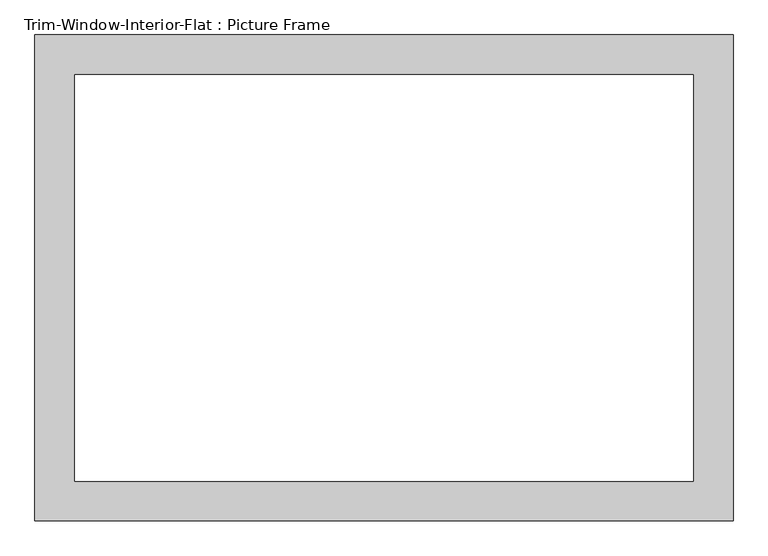
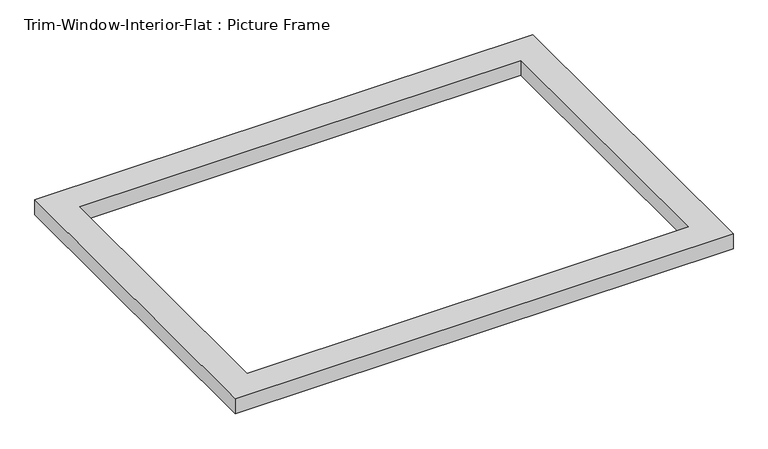
"""IFC4 building model written with IfcOpenShell, lengths in millimetres: proxy geometry, Trim-Window-Interior-Flat : Picture Frame."""

from ifc_helpers import new_model, si_unit, origin, origin_with_axes, place, context, project, spatial, polyline, outline, extrude, source, transform, mapped, element, save


def trim_window_interior_flat_picture_frame_6592d821(model_context):
    return source(origin(), model_context, "Body", "SweptSolid", [
        extrude(outline(polyline([(501.65, 44.45), (501.65, -654.05), (-501.65, -654.05), (-501.65, 44.45), (501.65, 44.45)]), holes=[polyline([(444.5, -12.7), (-444.5, -12.7), (-444.5, -596.9), (444.5, -596.9), (444.5, -12.7)])]), origin_with_axes(), (0.0, 0.0, 1.0), 31.75),
    ])


if __name__ == "__main__":
    model = new_model("IFC4")
    model_context = context("Model", 3, world=origin())
    ifc_project = project(units=[si_unit("LENGTHUNIT", "METRE", prefix="MILLI")], contexts=[model_context])
    site = spatial("IfcSite", under=ifc_project)
    building = spatial("IfcBuilding", under=site)
    placement = place(None, origin())
    trim_window_interior_flat_picture_frame_shape = trim_window_interior_flat_picture_frame_6592d821(model_context)
    element("IfcBuildingElementProxy", 1, Name="Trim-Window-Interior-Flat : Picture Frame", ObjectType="Trim-Window-Interior-Flat : Picture Frame", at=placement, inside=building, context=model_context, shape_type="MappedRepresentation", body=[
        mapped(trim_window_interior_flat_picture_frame_shape, transform((0.0, 0.0, 0.0), x_axis=(1.0, 0.0, 0.0), y_axis=(0.0, 1.0, 0.0), z_axis=(0.0, 0.0, 1.0))),
    ])
    save(model, "model.ifc")

# Revit data of these elements
# Type "Trim-Window-Interior-Flat : Picture Frame"
#   Trim Thickness_Picture Frame = 1.25"
#   Trim Width = 2.25"
#   Trim Thickness_with Sill = 0.75"
#   Sill Thickness = 1.25"
#   Opening Width [instance default] = 24"
#   Opening Height [instance default] = 36"
#   Default Elevation = 48"
#   Sill = no
#   Picture Frame = yes
#   Trim Material [instance default] = none
# Element 1 (IfcBuildingElementProxy, "Trim-Window-Interior-Flat : Picture Frame")
#   Opening Width = 36"
#   Opening Height = 24"
#   Trim Material = Wood - Stained
#   Materials on its faces: "Wood - Stained"
# Materials
#   "Wood - Stained": class "Wood", colour RGB 224 178 126, transparency 0, Cost = 0
